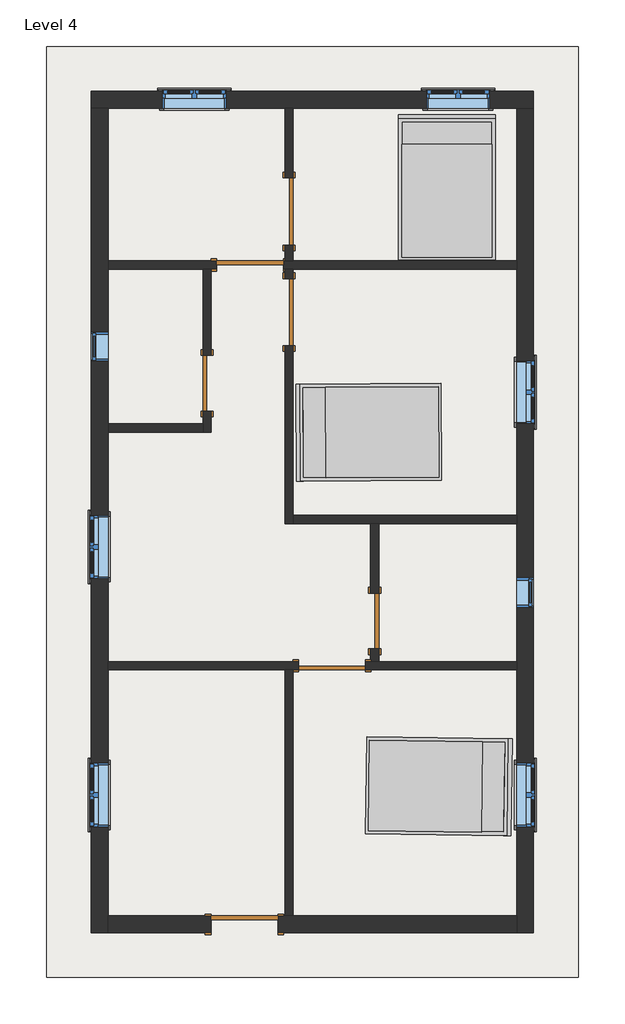
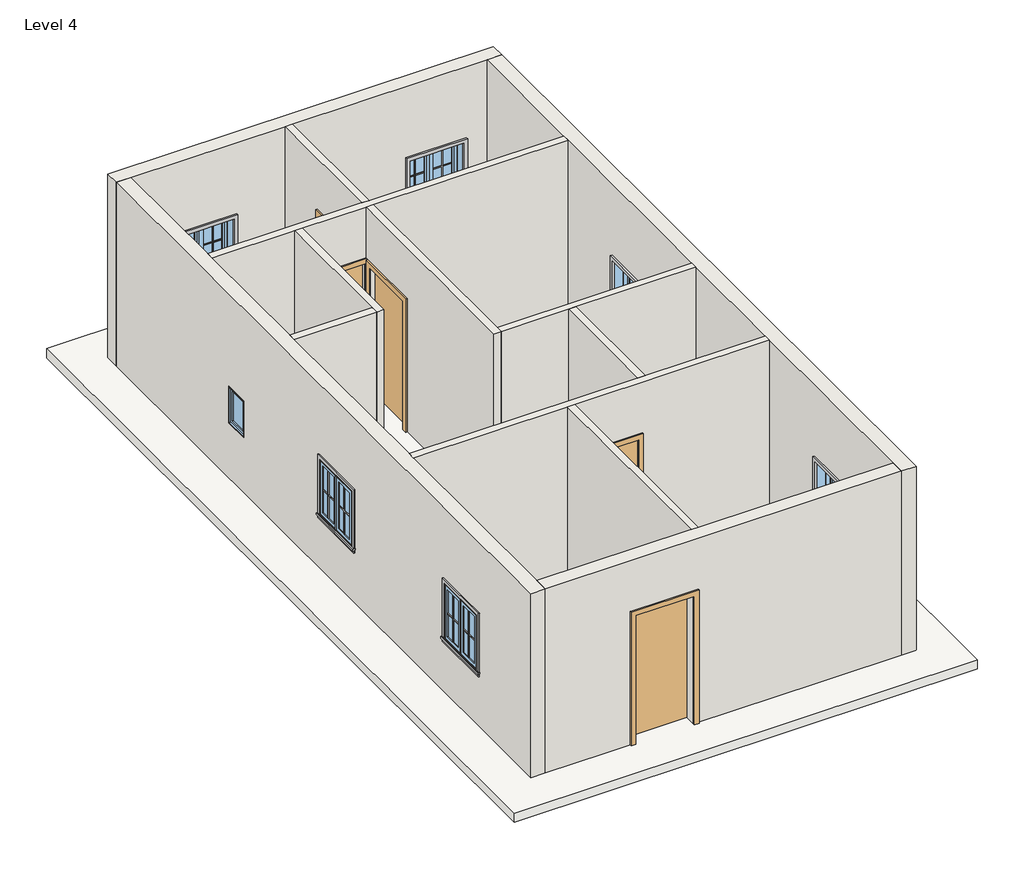
# One storey, incomplete: 24 proxies, 12 walls, 8 windows, 7 doors, 3 furniture elements, 1 roof.
"""IFC4 building model written with IfcOpenShell, lengths in millimetres."""

from ifc_helpers import new_model, si_unit, frame, origin, place, context, project, spatial, polyline, outline, extrude, faceted_brep, transform, mapped, element, save
from components import muntin_pattern_2x2_muntin_pattern_2x2_b3fe6957, muntin_pattern_2x2_muntin_pattern_2x2_3e0ecaf2, trim_window_exterior_flat_with_sill_41619996, trim_window_interior_flat_picture_frame_51c85655, door_d8f5dbb5, door_f2b275c1, door_e5f9f3c4, door_305aa2a5, door_0ca8825f, bed_17739_bed_17739_15c61121, window_aa618e30, window_339605e1

model = new_model("IFC4")

# Units and contexts
model_context = context("Model", 3, world=origin())
ifc_project = project(units=[si_unit("LENGTHUNIT", "METRE", prefix="MILLI")], contexts=[model_context])

# Site, building, storey
site = spatial("IfcSite", under=ifc_project)
building = spatial("IfcBuilding", under=site)
storey = spatial("IfcBuildingStorey", under=building, Name="Level 4", Elevation=6400.8)

# Proxies
placement = place(None, origin())
muntin_pattern_2x2_muntin_pattern_2x2_shape = muntin_pattern_2x2_muntin_pattern_2x2_b3fe6957(model_context)
element("IfcBuildingElementProxy", 1, Name="Muntin Pattern_2x2 : Muntin Pattern_2x2", ObjectType="Muntin Pattern_2x2 : Muntin Pattern_2x2", at=placement, inside=storey, context=model_context, shape_type="MappedRepresentation", body=[
    mapped(muntin_pattern_2x2_muntin_pattern_2x2_shape, transform((517.9959916, 6415.1185985, 7385.05), x_axis=(1.0, 0.0, 0.0), y_axis=(0.0, 1.0, 0.0), z_axis=(0.0, 0.0, 1.0))),
])
element("IfcBuildingElementProxy", 2, Name="Muntin Pattern_2x2 : Muntin Pattern_2x2", ObjectType="Muntin Pattern_2x2 : Muntin Pattern_2x2", at=placement, inside=storey, context=model_context, shape_type="MappedRepresentation", body=[
    mapped(muntin_pattern_2x2_muntin_pattern_2x2_shape, transform((-3079.2790084, 6415.1185985, 7385.05), x_axis=(1.0, 0.0, 0.0), y_axis=(0.0, 1.0, 0.0), z_axis=(0.0, 0.0, 1.0))),
])
element("IfcBuildingElementProxy", 3, Name="Muntin Pattern_2x2 : Muntin Pattern_2x2", ObjectType="Muntin Pattern_2x2 : Muntin Pattern_2x2", at=placement, inside=storey, context=model_context, shape_type="MappedRepresentation", body=[
    mapped(muntin_pattern_2x2_muntin_pattern_2x2_shape, transform((1751.4834916, 2536.8560985, 7385.05), x_axis=(0.0, -1.0, 0.0), y_axis=(1.0, 0.0, 0.0), z_axis=(0.0, 0.0, 1.0))),
])
element("IfcBuildingElementProxy", 4, Name="Muntin Pattern_2x2 : Muntin Pattern_2x2", ObjectType="Muntin Pattern_2x2 : Muntin Pattern_2x2", at=placement, inside=storey, context=model_context, shape_type="MappedRepresentation", body=[
    mapped(muntin_pattern_2x2_muntin_pattern_2x2_shape, transform((-4261.9665084, 0.0310985, 7385.05), x_axis=(0.0, 1.0, 0.0), y_axis=(-1.0, 0.0, 0.0), z_axis=(0.0, 0.0, 1.0))),
])
element("IfcBuildingElementProxy", 5, Name="Muntin Pattern_2x2 : Muntin Pattern_2x2", ObjectType="Muntin Pattern_2x2 : Muntin Pattern_2x2", at=placement, inside=storey, context=model_context, shape_type="MappedRepresentation", body=[
    mapped(muntin_pattern_2x2_muntin_pattern_2x2_shape, transform((-4261.9665084, -3381.3439015, 7385.05), x_axis=(0.0, 1.0, 0.0), y_axis=(-1.0, 0.0, 0.0), z_axis=(0.0, 0.0, 1.0))),
])
element("IfcBuildingElementProxy", 6, Name="Muntin Pattern_2x2 : Muntin Pattern_2x2", ObjectType="Muntin Pattern_2x2 : Muntin Pattern_2x2", at=placement, inside=storey, context=model_context, shape_type="MappedRepresentation", body=[
    mapped(muntin_pattern_2x2_muntin_pattern_2x2_shape, transform((1751.4834916, -2952.7189015, 7385.05), x_axis=(0.0, -1.0, 0.0), y_axis=(1.0, 0.0, 0.0), z_axis=(0.0, 0.0, 1.0))),
])
muntin_pattern_2x2_muntin_pattern_2x2_2_shape = muntin_pattern_2x2_muntin_pattern_2x2_3e0ecaf2(model_context)
element("IfcBuildingElementProxy", 7, Name="Muntin Pattern_2x2 : Muntin Pattern_2x2", ObjectType="Muntin Pattern_2x2 : Muntin Pattern_2x2", at=placement, inside=storey, context=model_context, shape_type="MappedRepresentation", body=[
    mapped(muntin_pattern_2x2_muntin_pattern_2x2_2_shape, transform((946.6209916, 6415.1185985, 7385.05), x_axis=(-1.0, 0.0, 0.0), y_axis=(0.0, -1.0, 0.0), z_axis=(0.0, 0.0, 1.0))),
])
element("IfcBuildingElementProxy", 8, Name="Muntin Pattern_2x2 : Muntin Pattern_2x2", ObjectType="Muntin Pattern_2x2 : Muntin Pattern_2x2", at=placement, inside=storey, context=model_context, shape_type="MappedRepresentation", body=[
    mapped(muntin_pattern_2x2_muntin_pattern_2x2_2_shape, transform((-2650.6540084, 6415.1185985, 7385.05), x_axis=(-1.0, 0.0, 0.0), y_axis=(0.0, -1.0, 0.0), z_axis=(0.0, 0.0, 1.0))),
])
element("IfcBuildingElementProxy", 9, Name="Muntin Pattern_2x2 : Muntin Pattern_2x2", ObjectType="Muntin Pattern_2x2 : Muntin Pattern_2x2", at=placement, inside=storey, context=model_context, shape_type="MappedRepresentation", body=[
    mapped(muntin_pattern_2x2_muntin_pattern_2x2_2_shape, transform((1751.4834916, 2108.2310985, 7385.05), x_axis=(0.0, 1.0, 0.0), y_axis=(-1.0, 0.0, 0.0), z_axis=(0.0, 0.0, 1.0))),
])
element("IfcBuildingElementProxy", 10, Name="Muntin Pattern_2x2 : Muntin Pattern_2x2", ObjectType="Muntin Pattern_2x2 : Muntin Pattern_2x2", at=placement, inside=storey, context=model_context, shape_type="MappedRepresentation", body=[
    mapped(muntin_pattern_2x2_muntin_pattern_2x2_2_shape, transform((-4261.9665084, 428.6560985, 7385.05), x_axis=(0.0, -1.0, 0.0), y_axis=(1.0, 0.0, 0.0), z_axis=(0.0, 0.0, 1.0))),
])
element("IfcBuildingElementProxy", 11, Name="Muntin Pattern_2x2 : Muntin Pattern_2x2", ObjectType="Muntin Pattern_2x2 : Muntin Pattern_2x2", at=placement, inside=storey, context=model_context, shape_type="MappedRepresentation", body=[
    mapped(muntin_pattern_2x2_muntin_pattern_2x2_2_shape, transform((-4261.9665084, -2952.7189015, 7385.05), x_axis=(0.0, -1.0, 0.0), y_axis=(1.0, 0.0, 0.0), z_axis=(0.0, 0.0, 1.0))),
])
element("IfcBuildingElementProxy", 12, Name="Muntin Pattern_2x2 : Muntin Pattern_2x2", ObjectType="Muntin Pattern_2x2 : Muntin Pattern_2x2", at=placement, inside=storey, context=model_context, shape_type="MappedRepresentation", body=[
    mapped(muntin_pattern_2x2_muntin_pattern_2x2_2_shape, transform((1751.4834916, -3381.3439015, 7385.05), x_axis=(0.0, 1.0, 0.0), y_axis=(-1.0, 0.0, 0.0), z_axis=(0.0, 0.0, 1.0))),
])
trim_window_exterior_flat_with_sill_shape = trim_window_exterior_flat_with_sill_41619996(model_context)
element("IfcBuildingElementProxy", 13, Name="Trim-Window-Exterior-Flat : with Sill", ObjectType="Trim-Window-Exterior-Flat : with Sill", at=placement, inside=storey, context=model_context, shape_type="MappedRepresentation", body=[
    mapped(trim_window_exterior_flat_with_sill_shape, transform((732.3084916, 6424.6435985, 8229.6), x_axis=(-1.0, 0.0, 0.0), y_axis=(0.0, 0.0, 1.0), z_axis=(0.0, 1.0, 0.0))),
])
element("IfcBuildingElementProxy", 14, Name="Trim-Window-Exterior-Flat : with Sill", ObjectType="Trim-Window-Exterior-Flat : with Sill", at=placement, inside=storey, context=model_context, shape_type="MappedRepresentation", body=[
    mapped(trim_window_exterior_flat_with_sill_shape, transform((-2864.9665084, 6424.6435985, 8229.6), x_axis=(-1.0, 0.0, 0.0), y_axis=(0.0, 0.0, 1.0), z_axis=(0.0, 1.0, 0.0))),
])
element("IfcBuildingElementProxy", 15, Name="Trim-Window-Exterior-Flat : with Sill", ObjectType="Trim-Window-Exterior-Flat : with Sill", at=placement, inside=storey, context=model_context, shape_type="MappedRepresentation", body=[
    mapped(trim_window_exterior_flat_with_sill_shape, transform((1761.0084916, 2322.5435985, 8229.6), x_axis=(0.0, 1.0, 0.0), y_axis=(0.0, 0.0, 1.0), z_axis=(1.0, 0.0, 0.0))),
])
element("IfcBuildingElementProxy", 16, Name="Trim-Window-Exterior-Flat : with Sill", ObjectType="Trim-Window-Exterior-Flat : with Sill", at=placement, inside=storey, context=model_context, shape_type="MappedRepresentation", body=[
    mapped(trim_window_exterior_flat_with_sill_shape, transform((-4271.4915084, 214.3435985, 8229.6), x_axis=(0.0, -1.0, 0.0), y_axis=(0.0, 0.0, 1.0), z_axis=(-1.0, 0.0, 0.0))),
])
element("IfcBuildingElementProxy", 17, Name="Trim-Window-Exterior-Flat : with Sill", ObjectType="Trim-Window-Exterior-Flat : with Sill", at=placement, inside=storey, context=model_context, shape_type="MappedRepresentation", body=[
    mapped(trim_window_exterior_flat_with_sill_shape, transform((-4271.4915084, -3167.0314015, 8229.6), x_axis=(0.0, -1.0, 0.0), y_axis=(0.0, 0.0, 1.0), z_axis=(-1.0, 0.0, 0.0))),
])
element("IfcBuildingElementProxy", 18, Name="Trim-Window-Exterior-Flat : with Sill", ObjectType="Trim-Window-Exterior-Flat : with Sill", at=placement, inside=storey, context=model_context, shape_type="MappedRepresentation", body=[
    mapped(trim_window_exterior_flat_with_sill_shape, transform((1761.0084916, -3167.0314015, 8229.6), x_axis=(0.0, 1.0, 0.0), y_axis=(0.0, 0.0, 1.0), z_axis=(1.0, 0.0, 0.0))),
])
trim_window_interior_flat_picture_frame_shape = trim_window_interior_flat_picture_frame_51c85655(model_context)
element("IfcBuildingElementProxy", 19, Name="Trim-Window-Interior-Flat : Picture Frame", ObjectType="Trim-Window-Interior-Flat : Picture Frame", at=placement, inside=storey, context=model_context, shape_type="MappedRepresentation", body=[
    mapped(trim_window_interior_flat_picture_frame_shape, transform((732.3084916, 6196.0435985, 8229.6), x_axis=(1.0, 0.0, 0.0), y_axis=(0.0, 0.0, 1.0), z_axis=(0.0, -1.0, 0.0))),
])
element("IfcBuildingElementProxy", 20, Name="Trim-Window-Interior-Flat : Picture Frame", ObjectType="Trim-Window-Interior-Flat : Picture Frame", at=placement, inside=storey, context=model_context, shape_type="MappedRepresentation", body=[
    mapped(trim_window_interior_flat_picture_frame_shape, transform((-2864.9665084, 6196.0435985, 8229.6), x_axis=(1.0, 0.0, 0.0), y_axis=(0.0, 0.0, 1.0), z_axis=(0.0, -1.0, 0.0))),
])
element("IfcBuildingElementProxy", 21, Name="Trim-Window-Interior-Flat : Picture Frame", ObjectType="Trim-Window-Interior-Flat : Picture Frame", at=placement, inside=storey, context=model_context, shape_type="MappedRepresentation", body=[
    mapped(trim_window_interior_flat_picture_frame_shape, transform((1532.4084916, 2322.5435985, 8229.6), x_axis=(0.0, -1.0, 0.0), y_axis=(0.0, 0.0, 1.0), z_axis=(-1.0, 0.0, 0.0))),
])
element("IfcBuildingElementProxy", 22, Name="Trim-Window-Interior-Flat : Picture Frame", ObjectType="Trim-Window-Interior-Flat : Picture Frame", at=placement, inside=storey, context=model_context, shape_type="MappedRepresentation", body=[
    mapped(trim_window_interior_flat_picture_frame_shape, transform((-4042.8915084, 214.3435985, 8229.6), x_axis=(0.0, 1.0, 0.0), y_axis=(0.0, 0.0, 1.0), z_axis=(1.0, 0.0, 0.0))),
])
element("IfcBuildingElementProxy", 23, Name="Trim-Window-Interior-Flat : Picture Frame", ObjectType="Trim-Window-Interior-Flat : Picture Frame", at=placement, inside=storey, context=model_context, shape_type="MappedRepresentation", body=[
    mapped(trim_window_interior_flat_picture_frame_shape, transform((-4042.8915084, -3167.0314015, 8229.6), x_axis=(0.0, 1.0, 0.0), y_axis=(0.0, 0.0, 1.0), z_axis=(1.0, 0.0, 0.0))),
])
element("IfcBuildingElementProxy", 24, Name="Trim-Window-Interior-Flat : Picture Frame", ObjectType="Trim-Window-Interior-Flat : Picture Frame", at=placement, inside=storey, context=model_context, shape_type="MappedRepresentation", body=[
    mapped(trim_window_interior_flat_picture_frame_shape, transform((1532.4084916, -3167.0314015, 8229.6), x_axis=(0.0, -1.0, 0.0), y_axis=(0.0, 0.0, 1.0), z_axis=(-1.0, 0.0, 0.0))),
])

# Doors
door_shape = door_d8f5dbb5(model_context)
element("IfcDoor", 25, ObjectType="Single-Flush : 30\" x 80\"", at=placement, inside=storey, context=model_context, shape_type="MappedRepresentation", body=[
    mapped(door_shape, transform((-404.3415084, -795.3064015, 6400.8), x_axis=(0.0, -1.0, 0.0), y_axis=(1.0, 0.0, 0.0), z_axis=(0.0, 0.0, 1.0))),
])
door_2_shape = door_f2b275c1(model_context)
element("IfcDoor", 26, ObjectType="Single-Flush : 30\" x 80\"", at=placement, inside=storey, context=model_context, shape_type="MappedRepresentation", body=[
    mapped(door_2_shape, transform((-2690.3415084, 2443.1935985, 6400.8), x_axis=(0.0, -1.0, 0.0), y_axis=(1.0, 0.0, 0.0), z_axis=(0.0, 0.0, 1.0))),
])
door_3_shape = door_e5f9f3c4(model_context)
element("IfcDoor", 27, ObjectType="Single-Flush : 36\" x 84\"", at=placement, inside=storey, context=model_context, shape_type="MappedRepresentation", body=[
    mapped(door_3_shape, transform((-2106.1415084, 4056.0935985, 6400.8), x_axis=(1.0, 0.0, 0.0), y_axis=(0.0, 1.0, 0.0), z_axis=(0.0, 0.0, 1.0))),
])
element("IfcDoor", 28, ObjectType="Single-Flush : 36\" x 84\"", at=placement, inside=storey, context=model_context, shape_type="MappedRepresentation", body=[
    mapped(door_3_shape, transform((-1572.7415084, 4786.3435985, 6400.8), x_axis=(0.0, -1.0, 0.0), y_axis=(1.0, 0.0, 0.0), z_axis=(0.0, 0.0, 1.0))),
])
element("IfcDoor", 29, ObjectType="Single-Flush : 36\" x 84\"", at=placement, inside=storey, context=model_context, shape_type="MappedRepresentation", body=[
    mapped(door_3_shape, transform((-988.5415084, -1404.9064015, 6400.8), x_axis=(-1.0, 0.0, 0.0), y_axis=(0.0, -1.0, 0.0), z_axis=(0.0, 0.0, 1.0))),
])
door_4_shape = door_305aa2a5(model_context)
element("IfcDoor", 30, ObjectType="Single-Flush : 36\" x 84\"", at=placement, inside=storey, context=model_context, shape_type="MappedRepresentation", body=[
    mapped(door_4_shape, transform((-1572.7415084, 3414.7435985, 6400.8), x_axis=(0.0, 1.0, 0.0), y_axis=(-1.0, 0.0, 0.0), z_axis=(0.0, 0.0, 1.0))),
])
door_5_shape = door_0ca8825f(model_context)
element("IfcDoor", 31, ObjectType="Single-Flush : 36\" x 84\"", at=placement, inside=storey, context=model_context, shape_type="MappedRepresentation", body=[
    mapped(door_5_shape, transform((-2182.3415084, -4929.1564015, 6400.8), x_axis=(1.0, 0.0, 0.0), y_axis=(0.0, 1.0, 0.0), z_axis=(0.0, 0.0, 1.0))),
])

# Furniture
bed_17739_bed_17739_shape = bed_17739_bed_17739_15c61121(model_context)
element("IfcFurniture", 32, ObjectType="Bed_17739 : Bed_17739", at=placement, inside=storey, context=model_context, shape_type="MappedRepresentation", body=[
    mapped(bed_17739_bed_17739_shape, transform((579.9084916, 5091.1435985, 6400.8), x_axis=(1.0, 0.0, 0.0), y_axis=(0.0, 1.0, 0.0), z_axis=(0.0, 0.0, 1.0))),
])
element("IfcFurniture", 33, ObjectType="Bed_17739 : Bed_17739", at=placement, inside=storey, context=model_context, shape_type="MappedRepresentation", body=[
    mapped(bed_17739_bed_17739_shape, transform((-461.4915084, 1776.4435985, 6400.8), x_axis=(-0.00529598194226197, 0.9999859761893001, 0.0), y_axis=(-0.9999859761893001, -0.00529598194226197, 0.0), z_axis=(0.0, 0.0, 1.0))),
])
element("IfcFurniture", 34, ObjectType="Bed_17739 : Bed_17739", at=placement, inside=storey, context=model_context, shape_type="MappedRepresentation", body=[
    mapped(bed_17739_bed_17739_shape, transform((445.2457081, -3048.1973462, 6400.8), x_axis=(-0.012781947661401841, -0.9999183075701641, 0.0), y_axis=(0.9999183075701641, -0.012781947661401841, 0.0), z_axis=(0.0, 0.0, 1.0))),
])

# Roof
element("IfcRoof", 35, ObjectType="Generic - 12\"", at=placement, inside=storey, context=model_context, shape_type="SweptSolid", body=[
    extrude(outline(polyline([(-4881.0915084, 7034.2435985), (2370.6084916, 7034.2435985), (2370.6084916, -5653.0564015), (-4881.0915084, -5653.0564015), (-4881.0915084, 7034.2435985)])), frame((0.0, 0.0, 6248.4), z_axis=(0.0, 0.0, 1.0), x_axis=(1.0, 0.0, 0.0)), (0.0, 0.0, 1.0), 152.4),
])

# Walls
element("IfcWall", 36, ObjectType="WALL4.5\"", at=placement, inside=storey, context=model_context, shape_type="Brep", body=[
    faceted_brep([(-1648.9415084, 3998.9435985, 8534.4), (-1648.9415084, 3998.9435985, 6400.8), (-1629.8915084, 3998.9435985, 6400.8), (-1515.5915084, 3998.9435985, 6400.8), (1532.4084916, 3998.9435985, 6400.8), (1532.4084916, 3998.9435985, 9448.8), (-1515.5915084, 3998.9435985, 9448.8), (-1629.8915084, 3998.9435985, 9448.8), (-2633.1915084, 3998.9435985, 9448.8), (-2747.4915084, 3998.9435985, 9448.8), (-4042.8915084, 3998.9435985, 9448.8), (-4042.8915084, 3998.9435985, 6400.8), (-2747.4915084, 3998.9435985, 6400.8), (-2633.1915084, 3998.9435985, 6400.8), (-2563.3415084, 3998.9435985, 6400.8), (-2563.3415084, 3998.9435985, 8534.4), (1532.4084916, 4113.2435985, 6400.8), (-1515.5915084, 4113.2435985, 6400.8), (-1629.8915084, 4113.2435985, 6400.8), (-1648.9415084, 4113.2435985, 6400.8), (-1648.9415084, 4113.2435985, 8534.4), (-2563.3415084, 4113.2435985, 8534.4), (-2563.3415084, 4113.2435985, 6400.8), (-4042.8915084, 4113.2435985, 6400.8), (-4042.8915084, 4113.2435985, 9448.8), (-1629.8915084, 4113.2435985, 9448.8), (-1515.5915084, 4113.2435985, 9448.8), (1532.4084916, 4113.2435985, 9448.8)], [[[0, 1, 2, 3, 4, 5, 6, 7, 8, 9, 10, 11, 12, 13, 14, 15]], [[16, 17, 18, 19, 20, 21, 22, 23, 24, 25, 26, 27]], [[4, 3, 2, 1, 19, 18, 17, 16]], [[14, 13, 12, 11, 23, 22]], [[5, 4, 16, 27]], [[11, 10, 24, 23]], [[20, 19, 1, 0]], [[21, 20, 0, 15]], [[22, 21, 15, 14]], [[10, 9, 8, 7, 6, 5, 27, 26, 25, 24]]]),
])
element("IfcWall", 37, ObjectType="WALL4.5\"", at=placement, inside=storey, context=model_context, shape_type="Brep", body=[
    faceted_brep([(-1629.8915084, 6196.0435985, 9448.8), (-1629.8915084, 6196.0435985, 6400.8), (-1629.8915084, 5243.5435985, 6400.8), (-1629.8915084, 5243.5435985, 8534.4), (-1629.8915084, 4329.1435985, 8534.4), (-1629.8915084, 4329.1435985, 6400.8), (-1629.8915084, 4113.2435985, 6400.8), (-1629.8915084, 4113.2435985, 9448.8), (-1515.5915084, 6196.0435985, 6400.8), (-1515.5915084, 6196.0435985, 9448.8), (-1515.5915084, 4113.2435985, 9448.8), (-1515.5915084, 4113.2435985, 6400.8), (-1515.5915084, 4329.1435985, 6400.8), (-1515.5915084, 4329.1435985, 8534.4), (-1515.5915084, 5243.5435985, 8534.4), (-1515.5915084, 5243.5435985, 6400.8)], [[[0, 1, 2, 3, 4, 5, 6, 7]], [[8, 9, 10, 11, 12, 13, 14, 15]], [[1, 8, 15, 2]], [[5, 12, 11, 6]], [[1, 0, 9, 8]], [[7, 6, 11, 10]], [[13, 12, 5, 4]], [[14, 13, 4, 3]], [[15, 14, 3, 2]], [[9, 0, 7, 10]]]),
    faceted_brep([(-1629.8915084, 531.8435985, 6400.8), (-1629.8915084, 531.8435985, 9448.8), (-1629.8915084, 3998.9435985, 9448.8), (-1629.8915084, 3998.9435985, 6400.8), (-1629.8915084, 3871.9435985, 6400.8), (-1629.8915084, 3871.9435985, 8534.4), (-1629.8915084, 2957.5435985, 8534.4), (-1629.8915084, 2957.5435985, 6400.8), (-1515.5915084, 531.8435985, 9448.8), (-1515.5915084, 531.8435985, 6400.8), (-1515.5915084, 646.1435985, 6400.8), (-1515.5915084, 2957.5435985, 6400.8), (-1515.5915084, 2957.5435985, 8534.4), (-1515.5915084, 3871.9435985, 8534.4), (-1515.5915084, 3871.9435985, 6400.8), (-1515.5915084, 3998.9435985, 6400.8), (-1515.5915084, 3998.9435985, 9448.8), (-1515.5915084, 646.1435985, 9448.8)], [[[0, 1, 2, 3, 4, 5, 6, 7]], [[8, 9, 10, 11, 12, 13, 14, 15, 16, 17]], [[9, 0, 7, 11, 10]], [[14, 4, 3, 15]], [[3, 2, 16, 15]], [[1, 0, 9, 8]], [[5, 4, 14, 13]], [[6, 5, 13, 12]], [[7, 6, 12, 11]], [[1, 8, 17, 16, 2]]]),
])
element("IfcWall", 38, ObjectType="WALL4.5\"", at=placement, inside=storey, context=model_context, shape_type="Brep", body=[
    faceted_brep([(-1515.5915084, 531.8435985, 6400.8), (-461.4915084, 531.8435985, 6400.8), (-347.1915084, 531.8435985, 6400.8), (1532.4084916, 531.8435985, 6400.8), (1532.4084916, 531.8435985, 9448.8), (-347.1915084, 531.8435985, 9448.8), (-461.4915084, 531.8435985, 9448.8), (-1515.5915084, 531.8435985, 9448.8), (-1515.5915084, 646.1435985, 6400.8), (-1515.5915084, 646.1435985, 9448.8), (1532.4084916, 646.1435985, 9448.8), (1532.4084916, 646.1435985, 6400.8)], [[[0, 1, 2, 3, 4, 5, 6, 7]], [[8, 9, 10, 11]], [[3, 2, 1, 0, 8, 11]], [[0, 7, 9, 8]], [[4, 3, 11, 10]], [[7, 6, 5, 4, 10, 9]]]),
])
element("IfcWall", 39, ObjectType="WALL4.5\"", at=placement, inside=storey, context=model_context, shape_type="Brep", body=[
    faceted_brep([(-2747.4915084, 2062.1935985, 8432.8), (-2747.4915084, 2062.1935985, 6400.8), (-2747.4915084, 1890.7435985, 6400.8), (-2747.4915084, 1776.4435985, 6400.8), (-2747.4915084, 1776.4435985, 9448.8), (-2747.4915084, 1890.7435985, 9448.8), (-2747.4915084, 3998.9435985, 9448.8), (-2747.4915084, 3998.9435985, 6400.8), (-2747.4915084, 2824.1935985, 6400.8), (-2747.4915084, 2824.1935985, 8432.8), (-2633.1915084, 1776.4435985, 6400.8), (-2633.1915084, 2062.1935985, 6400.8), (-2633.1915084, 2062.1935985, 8432.8), (-2633.1915084, 2824.1935985, 8432.8), (-2633.1915084, 2824.1935985, 6400.8), (-2633.1915084, 3998.9435985, 6400.8), (-2633.1915084, 3998.9435985, 9448.8), (-2633.1915084, 1776.4435985, 9448.8)], [[[0, 1, 2, 3, 4, 5, 6, 7, 8, 9]], [[10, 11, 12, 13, 14, 15, 16, 17]], [[8, 7, 15, 14]], [[3, 2, 1, 11, 10]], [[7, 6, 16, 15]], [[4, 3, 10, 17]], [[12, 11, 1, 0]], [[13, 12, 0, 9]], [[14, 13, 9, 8]], [[6, 5, 4, 17, 16]]]),
])
element("IfcWall", 40, ObjectType="WALL4.5\"", at=placement, inside=storey, context=model_context, shape_type="SweptSolid", body=[
    extrude(outline(polyline([(-2747.4915084, 1776.4435985), (-4042.8915084, 1776.4435985), (-4042.8915084, 1890.7435985), (-2747.4915084, 1890.7435985), (-2747.4915084, 1776.4435985)])), frame((0.0, 0.0, 6400.8), z_axis=(0.0, 0.0, 1.0), x_axis=(1.0, 0.0, 0.0)), (0.0, 0.0, 1.0), 3048.0),
])
element("IfcWall", 41, ObjectType="WALL4.5\"", at=placement, inside=storey, context=model_context, shape_type="SweptSolid", body=[
    extrude(outline(polyline([(-1176.3064015, 8432.8), (-1176.3064015, 6400.8), (-1347.7564015, 6400.8), (-1347.7564015, 9448.8), (531.8435985, 9448.8), (531.8435985, 6400.8), (-414.3064015, 6400.8), (-414.3064015, 8432.8), (-1176.3064015, 8432.8)])), frame((-461.4915084, 0.0, 0.0), z_axis=(1.0, 0.0, 0.0), x_axis=(0.0, 1.0, 0.0)), (0.0, 0.0, 1.0), 114.3),
])
element("IfcWall", 42, ObjectType="WALL4.5\"", at=placement, inside=storey, context=model_context, shape_type="Brep", body=[
    faceted_brep([(-4042.8915084, -1462.0564015, 6400.8), (-1629.8915084, -1462.0564015, 6400.8), (-1515.5915084, -1462.0564015, 6400.8), (-1445.7415084, -1462.0564015, 6400.8), (-1445.7415084, -1462.0564015, 8534.4), (-531.3415084, -1462.0564015, 8534.4), (-531.3415084, -1462.0564015, 6400.8), (1532.4084916, -1462.0564015, 6400.8), (1532.4084916, -1462.0564015, 9448.8), (-1515.5915084, -1462.0564015, 9448.8), (-1629.8915084, -1462.0564015, 9448.8), (-4042.8915084, -1462.0564015, 9448.8), (-1445.7415084, -1347.7564015, 8534.4), (-1445.7415084, -1347.7564015, 6400.8), (-4042.8915084, -1347.7564015, 6400.8), (-4042.8915084, -1347.7564015, 9448.8), (-461.4915084, -1347.7564015, 9448.8), (-347.1915084, -1347.7564015, 9448.8), (1532.4084916, -1347.7564015, 9448.8), (1532.4084916, -1347.7564015, 6400.8), (-347.1915084, -1347.7564015, 6400.8), (-461.4915084, -1347.7564015, 6400.8), (-531.3415084, -1347.7564015, 6400.8), (-531.3415084, -1347.7564015, 8534.4)], [[[0, 1, 2, 3, 4, 5, 6, 7, 8, 9, 10, 11]], [[12, 13, 14, 15, 16, 17, 18, 19, 20, 21, 22, 23]], [[14, 13, 3, 2, 1, 0]], [[22, 21, 20, 19, 7, 6]], [[8, 7, 19, 18]], [[0, 11, 15, 14]], [[4, 3, 13, 12]], [[5, 4, 12, 23]], [[6, 5, 23, 22]], [[11, 10, 9, 8, 18, 17, 16, 15]]]),
])
element("IfcWall", 43, ObjectType="WALL4.5\"", at=placement, inside=storey, context=model_context, shape_type="SweptSolid", body=[
    extrude(outline(polyline([(-1629.8915084, -4814.8564015), (-1629.8915084, -1462.0564015), (-1515.5915084, -1462.0564015), (-1515.5915084, -4814.8564015), (-1629.8915084, -4814.8564015)])), frame((0.0, 0.0, 6400.8), z_axis=(0.0, 0.0, 1.0), x_axis=(1.0, 0.0, 0.0)), (0.0, 0.0, 1.0), 3048.0),
])
element("IfcWall", 44, ObjectType="WALL9\"", at=placement, inside=storey, context=model_context, shape_type="Brep", body=[
    faceted_brep([(-4271.4915084, 6196.0435985, 6400.8), (-4042.8915084, 6196.0435985, 6400.8), (-1629.8915084, 6196.0435985, 6400.8), (-1515.5915084, 6196.0435985, 6400.8), (1532.4084916, 6196.0435985, 6400.8), (1761.0084916, 6196.0435985, 6400.8), (1761.0084916, 6196.0435985, 9448.8), (1532.4084916, 6196.0435985, 9448.8), (-1515.5915084, 6196.0435985, 9448.8), (-1629.8915084, 6196.0435985, 9448.8), (-4042.8915084, 6196.0435985, 9448.8), (-4271.4915084, 6196.0435985, 9448.8), (1164.1084916, 6196.0435985, 8229.6), (1164.1084916, 6196.0435985, 7315.2), (300.5084916, 6196.0435985, 7315.2), (300.5084916, 6196.0435985, 8229.6), (-2433.1665084, 6196.0435985, 8229.6), (-2433.1665084, 6196.0435985, 7315.2), (-3296.7665084, 6196.0435985, 7315.2), (-3296.7665084, 6196.0435985, 8229.6), (-4271.4915084, 6424.6435985, 6400.8), (-4271.4915084, 6424.6435985, 9448.8), (1761.0084916, 6424.6435985, 9448.8), (1761.0084916, 6424.6435985, 6400.8), (1164.1084916, 6424.6435985, 8229.6), (300.5084916, 6424.6435985, 8229.6), (300.5084916, 6424.6435985, 7315.2), (1164.1084916, 6424.6435985, 7315.2), (-2433.1665084, 6424.6435985, 8229.6), (-3296.7665084, 6424.6435985, 8229.6), (-3296.7665084, 6424.6435985, 7315.2), (-2433.1665084, 6424.6435985, 7315.2)], [[[0, 1, 2, 3, 4, 5, 6, 7, 8, 9, 10, 11], [12, 13, 14, 15], [16, 17, 18, 19]], [[20, 21, 22, 23], [24, 25, 26, 27], [28, 29, 30, 31]], [[5, 4, 3, 2, 1, 0, 20, 23]], [[6, 5, 23, 22]], [[0, 11, 21, 20]], [[13, 12, 24, 27]], [[14, 13, 27, 26]], [[15, 14, 26, 25]], [[12, 15, 25, 24]], [[17, 16, 28, 31]], [[18, 17, 31, 30]], [[19, 18, 30, 29]], [[16, 19, 29, 28]], [[11, 10, 9, 8, 7, 6, 22, 21]]]),
])
element("IfcWall", 45, ObjectType="WALL9\"", at=placement, inside=storey, context=model_context, shape_type="Brep", body=[
    faceted_brep([(1532.4084916, 6196.0435985, 6400.8), (1532.4084916, 4113.2435985, 6400.8), (1532.4084916, 3998.9435985, 6400.8), (1532.4084916, 646.1435985, 6400.8), (1532.4084916, 531.8435985, 6400.8), (1532.4084916, -1347.7564015, 6400.8), (1532.4084916, -1462.0564015, 6400.8), (1532.4084916, -4814.8564015, 6400.8), (1532.4084916, -5043.4564015, 6400.8), (1532.4084916, -5043.4564015, 9448.8), (1532.4084916, -4814.8564015, 9448.8), (1532.4084916, -1462.0564015, 9448.8), (1532.4084916, -1347.7564015, 9448.8), (1532.4084916, 531.8435985, 9448.8), (1532.4084916, 646.1435985, 9448.8), (1532.4084916, 3998.9435985, 9448.8), (1532.4084916, 4113.2435985, 9448.8), (1532.4084916, 6196.0435985, 9448.8), (1532.4084916, -611.1564015, 7924.8), (1532.4084916, -611.1564015, 7315.2), (1532.4084916, -204.7564015, 7315.2), (1532.4084916, -204.7564015, 7924.8), (1532.4084916, 1890.7435985, 8229.6), (1532.4084916, 1890.7435985, 7315.2), (1532.4084916, 2754.3435985, 7315.2), (1532.4084916, 2754.3435985, 8229.6), (1532.4084916, -3598.8314015, 8229.6), (1532.4084916, -3598.8314015, 7315.2), (1532.4084916, -2735.2314015, 7315.2), (1532.4084916, -2735.2314015, 8229.6), (1761.0084916, 6196.0435985, 6400.8), (1761.0084916, 6196.0435985, 9448.8), (1761.0084916, -5043.4564015, 9448.8), (1761.0084916, -5043.4564015, 6400.8), (1761.0084916, -611.1564015, 7924.8), (1761.0084916, -204.7564015, 7924.8), (1761.0084916, -204.7564015, 7315.2), (1761.0084916, -611.1564015, 7315.2), (1761.0084916, 1890.7435985, 8229.6), (1761.0084916, 2754.3435985, 8229.6), (1761.0084916, 2754.3435985, 7315.2), (1761.0084916, 1890.7435985, 7315.2), (1761.0084916, -3598.8314015, 8229.6), (1761.0084916, -2735.2314015, 8229.6), (1761.0084916, -2735.2314015, 7315.2), (1761.0084916, -3598.8314015, 7315.2)], [[[0, 1, 2, 3, 4, 5, 6, 7, 8, 9, 10, 11, 12, 13, 14, 15, 16, 17], [18, 19, 20, 21], [22, 23, 24, 25], [26, 27, 28, 29]], [[30, 31, 32, 33], [34, 35, 36, 37], [38, 39, 40, 41], [42, 43, 44, 45]], [[8, 7, 6, 5, 4, 3, 2, 1, 0, 30, 33]], [[0, 17, 31, 30]], [[9, 8, 33, 32]], [[19, 18, 34, 37]], [[20, 19, 37, 36]], [[21, 20, 36, 35]], [[18, 21, 35, 34]], [[23, 22, 38, 41]], [[24, 23, 41, 40]], [[25, 24, 40, 39]], [[22, 25, 39, 38]], [[27, 26, 42, 45]], [[28, 27, 45, 44]], [[29, 28, 44, 43]], [[26, 29, 43, 42]], [[17, 16, 15, 14, 13, 12, 11, 10, 9, 32, 31]]]),
])
element("IfcWall", 46, ObjectType="WALL9\"", at=placement, inside=storey, context=model_context, shape_type="Brep", body=[
    faceted_brep([(-4271.4915084, 6196.0435985, 6400.8), (-4271.4915084, -5043.4564015, 6400.8), (-4271.4915084, -5043.4564015, 9448.8), (-4271.4915084, 6196.0435985, 9448.8), (-4271.4915084, 3148.0435985, 7924.8), (-4271.4915084, 2741.6435985, 7924.8), (-4271.4915084, 2741.6435985, 7315.2), (-4271.4915084, 3148.0435985, 7315.2), (-4271.4915084, 646.1435985, 8229.6), (-4271.4915084, -217.4564015, 8229.6), (-4271.4915084, -217.4564015, 7315.2), (-4271.4915084, 646.1435985, 7315.2), (-4271.4915084, -2735.2314015, 8229.6), (-4271.4915084, -3598.8314015, 8229.6), (-4271.4915084, -3598.8314015, 7315.2), (-4271.4915084, -2735.2314015, 7315.2), (-4042.8915084, 6196.0435985, 6400.8), (-4042.8915084, 6196.0435985, 9448.8), (-4042.8915084, 4113.2435985, 9448.8), (-4042.8915084, 3998.9435985, 9448.8), (-4042.8915084, 1890.7435985, 9448.8), (-4042.8915084, 1776.4435985, 9448.8), (-4042.8915084, -1347.7564015, 9448.8), (-4042.8915084, -1462.0564015, 9448.8), (-4042.8915084, -4814.8564015, 9448.8), (-4042.8915084, -5043.4564015, 9448.8), (-4042.8915084, -5043.4564015, 6400.8), (-4042.8915084, -4814.8564015, 6400.8), (-4042.8915084, -1462.0564015, 6400.8), (-4042.8915084, -1347.7564015, 6400.8), (-4042.8915084, 1776.4435985, 6400.8), (-4042.8915084, 1890.7435985, 6400.8), (-4042.8915084, 3998.9435985, 6400.8), (-4042.8915084, 4113.2435985, 6400.8), (-4042.8915084, 3148.0435985, 7924.8), (-4042.8915084, 3148.0435985, 7315.2), (-4042.8915084, 2741.6435985, 7315.2), (-4042.8915084, 2741.6435985, 7924.8), (-4042.8915084, 646.1435985, 8229.6), (-4042.8915084, 646.1435985, 7315.2), (-4042.8915084, -217.4564015, 7315.2), (-4042.8915084, -217.4564015, 8229.6), (-4042.8915084, -2735.2314015, 8229.6), (-4042.8915084, -2735.2314015, 7315.2), (-4042.8915084, -3598.8314015, 7315.2), (-4042.8915084, -3598.8314015, 8229.6)], [[[0, 1, 2, 3], [4, 5, 6, 7], [8, 9, 10, 11], [12, 13, 14, 15]], [[16, 17, 18, 19, 20, 21, 22, 23, 24, 25, 26, 27, 28, 29, 30, 31, 32, 33], [34, 35, 36, 37], [38, 39, 40, 41], [42, 43, 44, 45]], [[1, 0, 16, 33, 32, 31, 30, 29, 28, 27, 26]], [[0, 3, 17, 16]], [[2, 1, 26, 25]], [[35, 34, 4, 7]], [[36, 35, 7, 6]], [[37, 36, 6, 5]], [[34, 37, 5, 4]], [[39, 38, 8, 11]], [[40, 39, 11, 10]], [[41, 40, 10, 9]], [[38, 41, 9, 8]], [[43, 42, 12, 15]], [[44, 43, 15, 14]], [[45, 44, 14, 13]], [[42, 45, 13, 12]], [[3, 2, 25, 24, 23, 22, 21, 20, 19, 18, 17]]]),
])
element("IfcWall", 47, ObjectType="WALL9\"", at=placement, inside=storey, context=model_context, shape_type="Brep", body=[
    faceted_brep([(-1725.1415084, -5043.4564015, 8534.4), (-1725.1415084, -5043.4564015, 6400.8), (1532.4084916, -5043.4564015, 6400.8), (1532.4084916, -5043.4564015, 9448.8), (-4042.8915084, -5043.4564015, 9448.8), (-4042.8915084, -5043.4564015, 6400.8), (-2639.5415084, -5043.4564015, 6400.8), (-2639.5415084, -5043.4564015, 8534.4), (1532.4084916, -4814.8564015, 6400.8), (-1515.5915084, -4814.8564015, 6400.8), (-1629.8915084, -4814.8564015, 6400.8), (-1725.1415084, -4814.8564015, 6400.8), (-1725.1415084, -4814.8564015, 8534.4), (-2639.5415084, -4814.8564015, 8534.4), (-2639.5415084, -4814.8564015, 6400.8), (-4042.8915084, -4814.8564015, 6400.8), (-4042.8915084, -4814.8564015, 9448.8), (-1629.8915084, -4814.8564015, 9448.8), (-1515.5915084, -4814.8564015, 9448.8), (1532.4084916, -4814.8564015, 9448.8)], [[[0, 1, 2, 3, 4, 5, 6, 7]], [[8, 9, 10, 11, 12, 13, 14, 15, 16, 17, 18, 19]], [[6, 5, 15, 14]], [[2, 1, 11, 10, 9, 8]], [[3, 2, 8, 19]], [[5, 4, 16, 15]], [[12, 11, 1, 0]], [[13, 12, 0, 7]], [[14, 13, 7, 6]], [[4, 3, 19, 18, 17, 16]]]),
])

# Windows
window_shape = window_aa618e30(model_context)
element("IfcWindow", 48, ObjectType="Fixed : 16\" x 24\"", at=placement, inside=storey, context=model_context, shape_type="MappedRepresentation", body=[
    mapped(window_shape, transform((1646.7084916, -446.0564015, 6400.8), x_axis=(0.0, -1.0, 0.0), y_axis=(1.0, 0.0, 0.0), z_axis=(0.0, 0.0, 1.0))),
])
element("IfcWindow", 49, ObjectType="Fixed : 16\" x 24\"", at=placement, inside=storey, context=model_context, shape_type="MappedRepresentation", body=[
    mapped(window_shape, transform((-4157.1915084, 2982.9435985, 6400.8), x_axis=(0.0, 1.0, 0.0), y_axis=(-1.0, 0.0, 0.0), z_axis=(0.0, 0.0, 1.0))),
])
window_2_shape = window_339605e1(model_context)
element("IfcWindow", 50, ObjectType="Window-Casement-Double : 34\" x 36\"", at=placement, inside=storey, context=model_context, shape_type="MappedRepresentation", body=[
    mapped(window_2_shape, transform((732.3084916, 6310.3435985, 6400.8), x_axis=(1.0, 0.0, 0.0), y_axis=(0.0, 1.0, 0.0), z_axis=(0.0, 0.0, 1.0))),
])
element("IfcWindow", 51, ObjectType="Window-Casement-Double : 34\" x 36\"", at=placement, inside=storey, context=model_context, shape_type="MappedRepresentation", body=[
    mapped(window_2_shape, transform((-2864.9665084, 6310.3435985, 6400.8), x_axis=(1.0, 0.0, 0.0), y_axis=(0.0, 1.0, 0.0), z_axis=(0.0, 0.0, 1.0))),
])
element("IfcWindow", 52, ObjectType="Window-Casement-Double : 34\" x 36\"", at=placement, inside=storey, context=model_context, shape_type="MappedRepresentation", body=[
    mapped(window_2_shape, transform((1646.7084916, 2322.5435985, 6400.8), x_axis=(0.0, -1.0, 0.0), y_axis=(1.0, 0.0, 0.0), z_axis=(0.0, 0.0, 1.0))),
])
element("IfcWindow", 53, ObjectType="Window-Casement-Double : 34\" x 36\"", at=placement, inside=storey, context=model_context, shape_type="MappedRepresentation", body=[
    mapped(window_2_shape, transform((-4157.1915084, 214.3435985, 6400.8), x_axis=(0.0, 1.0, 0.0), y_axis=(-1.0, 0.0, 0.0), z_axis=(0.0, 0.0, 1.0))),
])
element("IfcWindow", 54, ObjectType="Window-Casement-Double : 34\" x 36\"", at=placement, inside=storey, context=model_context, shape_type="MappedRepresentation", body=[
    mapped(window_2_shape, transform((-4157.1915084, -3167.0314015, 6400.8), x_axis=(0.0, 1.0, 0.0), y_axis=(-1.0, 0.0, 0.0), z_axis=(0.0, 0.0, 1.0))),
])
element("IfcWindow", 55, ObjectType="Window-Casement-Double : 34\" x 36\"", at=placement, inside=storey, context=model_context, shape_type="MappedRepresentation", body=[
    mapped(window_2_shape, transform((1646.7084916, -3167.0314015, 6400.8), x_axis=(0.0, -1.0, 0.0), y_axis=(1.0, 0.0, 0.0), z_axis=(0.0, 0.0, 1.0))),
])

save(model, "model.ifc")

# Revit data of these elements
# Type "Muntin Pattern_2x2 : Muntin Pattern_2x2"
#   Width [instance default] = 4' - 0"
#   Thickness = 0' - 0 1/2"
#   Height [instance default] = 4' - 0"
#   Distance = 0' - 0 3/4"
#   Interior Material [instance default] = none
#   Exterior Material [instance default] = none
#   Default Elevation = 0
# Type "Trim-Window-Exterior-Flat : with Sill"
#   Trim Width = 0' - 2 1/4"
#   Trim Thickness_Picture Frame = 0' - 1 1/4"
#   Trim Thickness_with Sill = 0' - 0 3/4"
#   Sill Thickness = 0' - 1 1/4"
#   Opening Width [instance default] = 2' - 0"
#   Opening Height [instance default] = 3' - 0"
#   Default Elevation = 4' - 0"
#   Sill = yes
#   Picture Frame = no
#   Trim Material [instance default] = none
# Type "Trim-Window-Interior-Flat : Picture Frame"
#   Trim Thickness_Picture Frame = 0' - 1 1/4"
#   Trim Width = 0' - 2 1/4"
#   Trim Thickness_with Sill = 0' - 0 3/4"
#   Sill Thickness = 0' - 1 1/4"
#   Opening Width [instance default] = 2' - 0"
#   Opening Height [instance default] = 3' - 0"
#   Default Elevation = 4' - 0"
#   Sill = no
#   Picture Frame = yes
#   Trim Material [instance default] = none
# Type "Single-Flush : 30\" x 80\""
#   Type Mark = "5"
#   Construction Type Id = "MDOOR"
#   Assembly Code = "C1020"
#   Analytic Construction = "Metal"
#   Thickness = 0' - 2"
#   Heat Transfer Coefficient (U) = 0.651978 BTU/(h·ft²·°F)
#   Height = 6' - 8"
#   Trim Projection Ext = 0' - 1"
#   Trim Projection Int = 0' - 1"
#   Trim Width = 0' - 3"
#   Width = 2' - 6"
#   Define Thermal Properties by = 1
#   Define Thermal Properties by = 1
#   Door Material = Door - Panel
#   Frame Material = Door - Frame
#   Visual Light Transmittance = 0
#   Solar Heat Gain Coefficient = 0
#   Function = (empty or 0)
#   Wall Closure = (empty or 0)
# Type "Single-Flush : 36\" x 84\""
#   Type Mark = "1"
#   Construction Type Id = "MDOOR"
#   Assembly Code = "C1020"
#   Analytic Construction = "Metal"
#   Thickness = 0' - 2"
#   Heat Transfer Coefficient (U) = 0.651978 BTU/(h·ft²·°F)
#   Height = 7' - 0"
#   Trim Projection Ext = 0' - 1"
#   Trim Projection Int = 0' - 1"
#   Trim Width = 0' - 3"
#   Width = 3' - 0"
#   Define Thermal Properties by = 1
#   Define Thermal Properties by = 1
#   Door Material = Door - Panel
#   Frame Material = Door - Frame
#   Visual Light Transmittance = 0
#   Solar Heat Gain Coefficient = 0
#   Function = (empty or 0)
#   Wall Closure = (empty or 0)
# Type "Bed_17739 : Bed_17739"
#   Default Elevation = 0
# Type "Generic - 12\""
#   Assembly Code = "B1020"
#   Layers, outside or top first: 0' - 6" no material (function 1)
# Type "WALL4.5\""
#   Assembly Code = "B2010"
#   Layers, outside or top first: 0' - 4 1/2" no material (function 1)
# Type "WALL9\""
#   Assembly Code = "B2010"
#   Layers, outside or top first: 0' - 9" no material (function 1)
# Type "Fixed : 16\" x 24\""
#   Type Mark = "4"
#   Construction Type Id = "GSP4R"
#   Assembly Code = "B2020100"
#   Analytic Construction = "1/8 in Pilkington single glazing"
#   Visual Light Transmittance = 0.9
#   Solar Heat Gain Coefficient = 0.78
#   Heat Transfer Coefficient (U) = 0.6496 BTU/(h·ft²·°F)
#   Height = 2' - 0"
#   Default Sill Height = 3' - 0"
#   Width = 1' - 4"
#   Window Inset = 0' - 0 3/4"
#   Define Thermal Properties by = 1
#   Define Thermal Properties by = 1
#   Glass Pane Material = Glass
#   Sash Material = Sash
#   Wall Closure = (empty or 0)
# Type "Window-Casement-Double : 34\" x 36\""
#   Type Mark = "14"
#   Fire Rating = "0.5h"
#   Assembly Code = "B2020100"
#   Analytic Construction = "Double glazing - domestic"
#   Frame Extension [instance default] = 0' - 0 1/4"
#   Window Inset [instance default] = 0' - 0"
#   Wall Thickness [instance default] = 0' - 6"
#   Interior Wall Closure [instance default] = 0' - 2 1/4"
#   Half Width = 1' - 5"
#   Visual Light Transmittance = 0.81
#   Thermal Resistance (R) = 1.8146 (h·ft²·°F)/BTU
#   Solar Heat Gain Coefficient = 0.76
#   Rough Width = 2' - 10 1/2"
#   Rough Height = 3' - 0 1/2"
#   Height = 3' - 0"
#   Heat Transfer Coefficient (U) = 0.5511 BTU/(h·ft²·°F)
#   Exterior Wall Closure [instance default] = 0' - 1 1/4"
#   Extension Jamb [instance default] = 0' - 2 1/4"
#   Default Sill Height = 3' - 0"
#   Width = 2' - 10"
#   Define Thermal Properties by = 0
#   Muntin Visibility = yes
#   Interior Trim Visibility [instance default] = yes
#   Exterior Trim Visibility [instance default] = yes
#   Extension Jamb Visibility [instance default] = yes
#   Interior Trim Material = Wood - Stained
#   Muntin Pattern = Muntin Pattern_2x2 : Muntin Pattern_2x2
#   Interior Trim = Trim-Window-Interior-Flat : Picture Frame
#   Interior Frame Material = Wood - Stained
#   Glass Panel Material = Glass
#   Exterior Trim Material = Clad - White
#   Exterior Trim = Trim-Window-Exterior-Flat : with Sill
#   Exterior Frame Material = Clad - White
#   Wall Closure = (empty or 0)
# Elements 1, 2, 3, 4, 5, 6, 7, 8, 9, 10, 11, 12 (IfcBuildingElementProxy, "Muntin Pattern_2x2 : Muntin Pattern_2x2")
#   Width = 0' - 11 5/8"
#   Height = 2' - 6 1/2"
#   Interior Material = Wood - Stained
#   Exterior Material = Clad - White
#   Phase Created = New Construction
#   Materials on its faces: "Clad - White", "Wood - Stained"
# Elements 13, 14, 15, 16, 17, 18 (IfcBuildingElementProxy, "Trim-Window-Exterior-Flat : with Sill")
#   Opening Width = 2' - 10"
#   Opening Height = 3' - 0"
#   Trim Material = Clad - White
#   Phase Created = New Construction
#   Materials on its faces: "Clad - White"
# Elements 19, 20, 21, 22, 23, 24 (IfcBuildingElementProxy, "Trim-Window-Interior-Flat : Picture Frame")
#   Opening Width = 2' - 10"
#   Opening Height = 3' - 0"
#   Trim Material = Wood - Stained
#   Phase Created = New Construction
#   Materials on its faces: "Wood - Stained"
# Elements 25, 26 (IfcDoor, "Single-Flush : 30\" x 80\"")
#   Phase Created = New Construction
#   Materials on its faces: "Door - Frame", "Door - Panel"
# Elements 27, 28, 29, 30, 31 (IfcDoor, "Single-Flush : 36\" x 84\"")
#   Phase Created = New Construction
#   Materials on its faces: "Door - Frame", "Door - Panel"
# Elements 32, 33, 34 (IfcFurniture, "Bed_17739 : Bed_17739")
#   Phase Created = New Construction
#   Materials on its faces: "legs", "sheets", "bed frame", "Blanket"
# Element 35 (IfcRoof, "Generic - 12\"")
#   built-in parameter 1001705 = 21 (stored number, unit not read)
#   built-in parameter 1001701 = -0.5 (stored number, unit not read)
#   built-in parameter 1001710 = 33615
#   Phase Created = New Construction
#   Materials on its faces: "Default Roof"
# Elements 36, 37, 38, 39, 40, 41, 42, 43 (IfcWall, "WALL4.5\"")
#   Top Offset = 0' - 0"
#   Base Offset = 0' - 0"
#   Unconnected Height = 10' - 0"
#   wall height = 10' - 0"
#   Phase Created = New Construction
#   Base Constraint = Level 4
#   Materials on its faces: "Default Wall"
# Elements 44, 45, 46, 47 (IfcWall, "WALL9\"")
#   Top Offset = 0' - 0"
#   Base Offset = 0' - 0"
#   Unconnected Height = 10' - 0"
#   wall height = 10' - 0"
#   Phase Created = New Construction
#   Base Constraint = Level 4
#   Materials on its faces: "Default Wall", "Brick, Common"
# Element 48 (IfcWindow, "Fixed : 16\" x 24\"")
#   Mark = "17"
#   Phase Created = New Construction
#   Materials on its faces: "Sash", "Glass"
# Element 49 (IfcWindow, "Fixed : 16\" x 24\"")
#   Mark = "18"
#   Phase Created = New Construction
#   Materials on its faces: "Sash", "Glass"
# Element 50 (IfcWindow, "Window-Casement-Double : 34\" x 36\"")
#   Mark = "19"
#   Window Inset = 0' - 0"
#   Interior Wall Closure = 0' - 2 1/4"
#   Frame Extension = 0' - 0 1/4"
#   Exterior Wall Closure = 0' - 1 1/4"
#   Interior Trim Visibility = yes
#   Exterior Trim Visibility = yes
#   Phase Created = New Construction
#   Materials on its faces: "Wood - Stained", "Glass", "Clad - White"
# Element 51 (IfcWindow, "Window-Casement-Double : 34\" x 36\"")
#   Mark = "20"
#   Window Inset = 0' - 0"
#   Interior Wall Closure = 0' - 2 1/4"
#   Frame Extension = 0' - 0 1/4"
#   Exterior Wall Closure = 0' - 1 1/4"
#   Interior Trim Visibility = yes
#   Exterior Trim Visibility = yes
#   Phase Created = New Construction
#   Materials on its faces: "Wood - Stained", "Glass", "Clad - White"
# Element 52 (IfcWindow, "Window-Casement-Double : 34\" x 36\"")
#   Mark = "21"
#   Window Inset = 0' - 0"
#   Interior Wall Closure = 0' - 2 1/4"
#   Frame Extension = 0' - 0 1/4"
#   Exterior Wall Closure = 0' - 1 1/4"
#   Interior Trim Visibility = yes
#   Exterior Trim Visibility = yes
#   Phase Created = New Construction
#   Materials on its faces: "Wood - Stained", "Glass", "Clad - White"
# Element 53 (IfcWindow, "Window-Casement-Double : 34\" x 36\"")
#   Mark = "22"
#   Window Inset = 0' - 0"
#   Interior Wall Closure = 0' - 2 1/4"
#   Frame Extension = 0' - 0 1/4"
#   Exterior Wall Closure = 0' - 1 1/4"
#   Interior Trim Visibility = yes
#   Exterior Trim Visibility = yes
#   Phase Created = New Construction
#   Materials on its faces: "Wood - Stained", "Glass", "Clad - White"
# Element 54 (IfcWindow, "Window-Casement-Double : 34\" x 36\"")
#   Mark = "23"
#   Window Inset = 0' - 0"
#   Interior Wall Closure = 0' - 2 1/4"
#   Frame Extension = 0' - 0 1/4"
#   Exterior Wall Closure = 0' - 1 1/4"
#   Interior Trim Visibility = yes
#   Exterior Trim Visibility = yes
#   Phase Created = New Construction
#   Materials on its faces: "Wood - Stained", "Glass", "Clad - White"
# Element 55 (IfcWindow, "Window-Casement-Double : 34\" x 36\"")
#   Mark = "24"
#   Window Inset = 0' - 0"
#   Interior Wall Closure = 0' - 2 1/4"
#   Frame Extension = 0' - 0 1/4"
#   Exterior Wall Closure = 0' - 1 1/4"
#   Interior Trim Visibility = yes
#   Exterior Trim Visibility = yes
#   Phase Created = New Construction
#   Materials on its faces: "Wood - Stained", "Glass", "Clad - White"
# Materials
#   "Door - Panel": class "Wood", colour RGB 210 159 95, transparency 0, Cost = 0
#   "Door - Frame": colour RGB 118 70 51, transparency 0, Cost = 0
#   "Glass": class "Glass", colour RGB 0 128 192, transparency 0.75, Description = "Soda Lime Glass", Cost = 0
#   "Sash": class "Wood", colour RGB 224 178 126, transparency 0, Cost = 0
#   "Wood - Stained": class "Wood", colour RGB 224 178 126, transparency 0, Cost = 0
#   "Clad - White": class "Wood", colour RGB 242 242 238, transparency 0, Cost = 0
#   "legs": colour RGB 90 73 37, transparency 0, Cost = 0
#   "sheets": colour RGB 200 195 176, transparency 0, Cost = 0
#   "bed frame": colour RGB 90 73 37, transparency 0, Cost = 0
#   "Blanket": class "System", colour RGB 59 0 1, transparency 0, Cost = 0
#   "Default Roof": colour RGB 88 101 114, transparency 0, Cost = 0
#   "Default Wall": colour RGB 128 128 128, transparency 0, Cost = 0
#   "Brick, Common": class "Masonry", colour RGB 170 98 104, transparency 0, Description = "Common brick", Cost = 0
